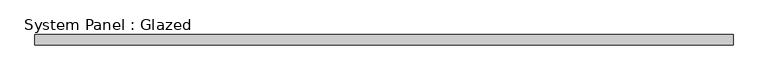
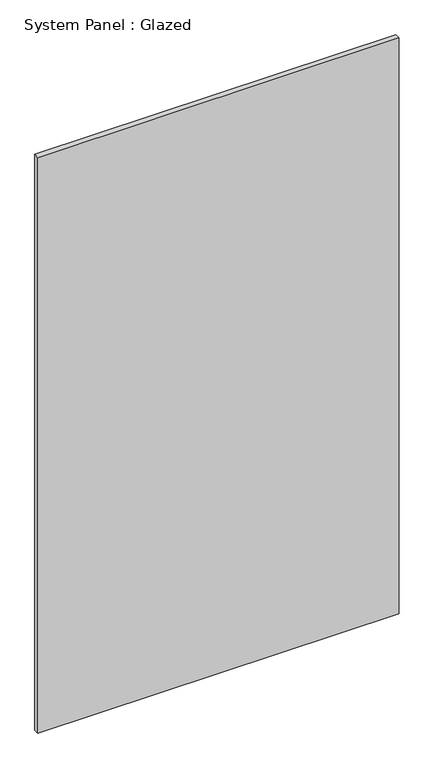
"""IFC4 building model written with IfcOpenShell, lengths in millimetres: plate geometry, System Panel : Glazed."""

from ifc_helpers import new_model, si_unit, origin, origin_with_axes, place, context, project, spatial, polyline, outline, extrude, source, transform, mapped, element, save


def system_panel_glazed_6b5a73aa(model_context):
    return source(origin(), model_context, "Body", "SweptSolid", [
        extrude(outline(polyline([(866.775, -44.45), (-866.775, -44.45), (-866.775, -19.05), (866.775, -19.05), (866.775, -44.45)])), origin_with_axes(), (0.0, 0.0, 1.0), 2921.0),
    ])


if __name__ == "__main__":
    model = new_model("IFC4")
    model_context = context("Model", 3, world=origin())
    ifc_project = project(units=[si_unit("LENGTHUNIT", "METRE", prefix="MILLI")], contexts=[model_context])
    site = spatial("IfcSite", under=ifc_project)
    building = spatial("IfcBuilding", under=site)
    placement = place(None, origin())
    system_panel_glazed_shape = system_panel_glazed_6b5a73aa(model_context)
    element("IfcPlate", 1, ObjectType="System Panel : Glazed", at=placement, inside=building, context=model_context, shape_type="MappedRepresentation", body=[
        mapped(system_panel_glazed_shape, transform((0.0, 0.0, 0.0), x_axis=(1.0, 0.0, 0.0), y_axis=(0.0, 1.0, 0.0), z_axis=(0.0, 0.0, 1.0))),
    ])
    save(model, "model.ifc")

# Revit data of these elements
# Type "System Panel : Glazed"
#   Construction Type Id = "GSP4R"
#   Analytic Construction = "1/8 in Pilkington single glazing"
#   Visual Light Transmittance = 0.9
#   Solar Heat Gain Coefficient = 0.86
#   Heat Transfer Coefficient (U) = 1.18115 BTU/(h·ft²·°F)
# Element 1 (IfcPlate, "System Panel : Glazed")
#   Materials on its faces: "Glass"
# Materials
#   "Glass": class "Glass", colour RGB 0 128 192, transparency 0.75, Description = "Soda Lime Glass", Cost = 0
